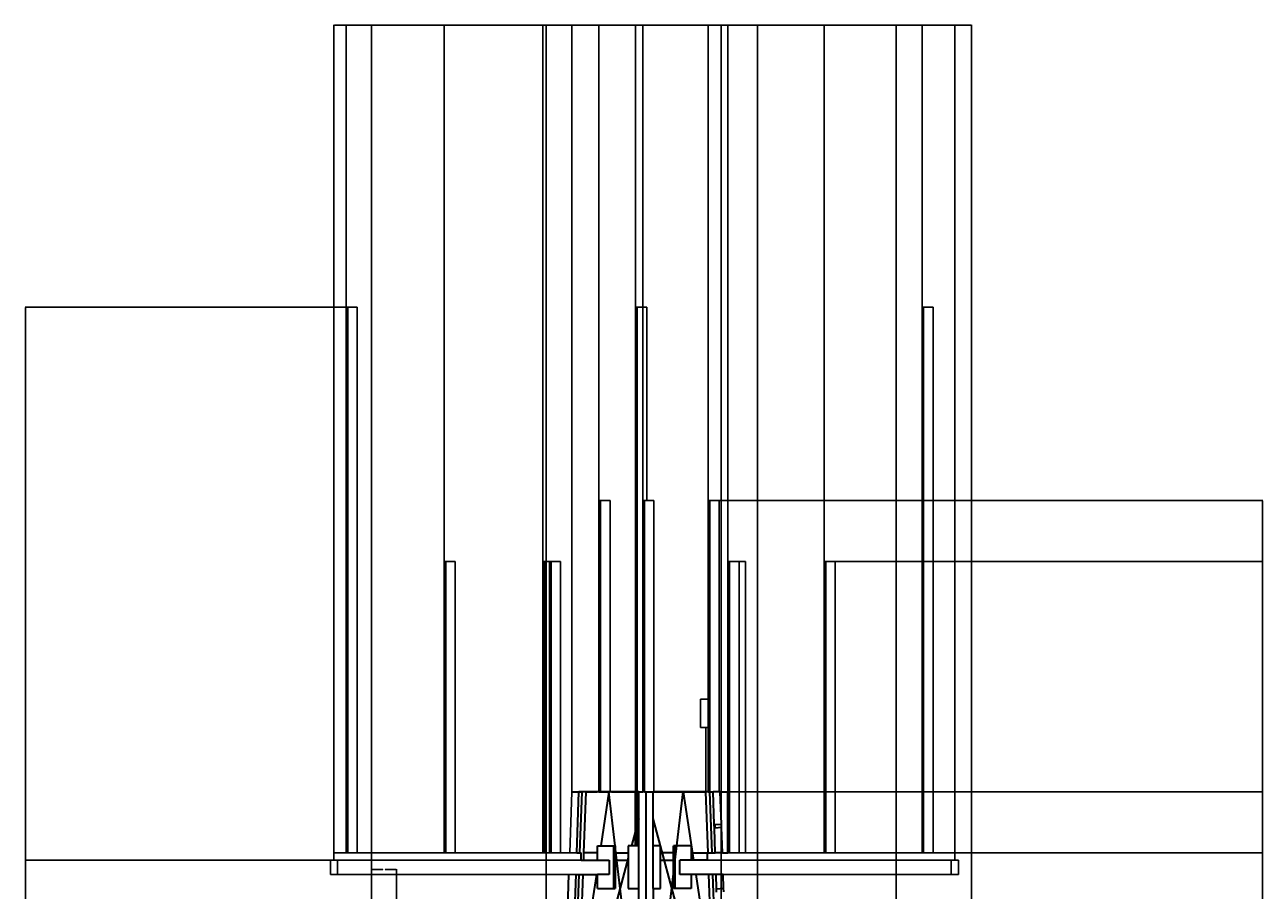
# Model space of a CAD drawing. Units: inches. Extents: x 3780 to 4301, y 1637 to 4224.
# Tile 8 of 8: x 3781 to 4301, y 3860 to 4224. Entities that reach past the tile are written whole.
import ezdxf

# ---------------------------------------------------------------- set-up
doc = ezdxf.new("R2010")
doc.units = ezdxf.units.IN
for name, color, linetype, lineweight in [('A-ANNO-DIMS', 2, 'Continuous', 18), ('E-COMM-ANTN', 4, 'Continuous', 25), ('S-TOWR', 7, 'Continuous', 35)]:
    doc.layers.add(name, color=color, linetype=linetype, lineweight=lineweight)
doc.styles.get("Standard").update_dxf_attribs({"font": 'arial.ttf'})
doc.dimstyles.get("Standard").update_dxf_attribs({"dimtxt": 0.18, "dimasz": 0.18, "dimexe": 0.18, "dimexo": 0.0625, "dimgap": 0.09, "dimtad": 0, "dimtih": 1, "dimtoh": 1, "dimdec": 4, "dimzin": 0, "dimdsep": 46, "dimtxsty": 'Standard', "dimcen": 0.09, "dimadec": 0, "dimazin": 0, "dimtfac": 1, "dimtdec": 4, "dimtofl": 0, "dimtmove": 0, "dimatfit": 3, "dimfxl": 1, "dimtolj": 1, "dimtzin": 0, "dimarcsym": 0})

# ---------------------------------------------------------------- blocks, each defined once
blk = doc.blocks.new('*D8')
at = {"layer": 'A-ANNO-DIMS', "color": 0, "lineweight": -2, "transparency": 16777216}
for p, q in [((3926.23, 3844.62), (3926.23, 3869.04)), ((3926.41, 3868.86), (3931, 3868.86)), ((3936.62, 3868.86), (3932.03, 3868.86)), ((3936.8, 3844.62), (3936.8, 3869.04))]:
    blk.add_line(p, q, dxfattribs=at)
at = {"layer": 'A-ANNO-DIMS', "color": 0, "transparency": 16777216}
for points in [[(3926.41, 3868.89), (3926.41, 3868.83), (3926.23, 3868.86)], [(3936.62, 3868.89), (3936.62, 3868.83), (3936.8, 3868.86)]]:
    blk.add_solid(points, dxfattribs=at)
at = {"layer": 'Defpoints', "color": 0, "transparency": 16777216}
for p in [(3936.8, 3868.86), (3926.23, 3844.56), (3936.8, 3844.56)]:
    blk.add_point(p, dxfattribs=at)
at = {"layer": 'A-ANNO-DIMS', "color": 0, "transparency": 16777216, "insert": (3931.51, 3868.86), "char_height": 0.18, "attachment_point": 5}
blk.add_mtext('\\A1;11 TYP.', dxfattribs=at)
blk = doc.blocks.new('*D11')
at = {"layer": 'A-ANNO-DIMS', "color": 0, "lineweight": -2, "transparency": 16777216}
for p, q in [((3916.19, 4105.28), (3780.66, 4105.28)), ((3780.84, 4105.1), (3780.84, 2930.44)), ((3780.84, 1755.43), (3780.84, 2930.08)), ((3934.09, 1755.25), (3780.66, 1755.25))]:
    blk.add_line(p, q, dxfattribs=at)
at = {"layer": 'A-ANNO-DIMS', "color": 0, "transparency": 16777216}
for points in [[(3780.81, 4105.1), (3780.87, 4105.1), (3780.84, 4105.28)], [(3780.81, 1755.43), (3780.87, 1755.43), (3780.84, 1755.25)]]:
    blk.add_solid(points, dxfattribs=at)
at = {"layer": 'Defpoints', "color": 0, "transparency": 16777216}
for p in [(3780.84, 4105.28), (3916.25, 4105.28), (3934.15, 1755.25)]:
    blk.add_point(p, dxfattribs=at)
at = {"layer": 'A-ANNO-DIMS', "color": 0, "transparency": 16777216, "insert": (3780.84, 2930.26), "char_height": 0.18, "attachment_point": 5}
blk.add_mtext('\\A1;2350', dxfattribs=at)
blk = doc.blocks.new('*D21')
at = {"layer": 'A-ANNO-DIMS', "color": 0, "lineweight": -2, "transparency": 16777216}
for p, q in [((4010.55, 3901.46), (4300.89, 3901.46)), ((4300.71, 3901.28), (4300.71, 3685.65)), ((4300.71, 3469.64), (4300.71, 3685.28)), ((4044.72, 3469.46), (4300.89, 3469.46))]:
    blk.add_line(p, q, dxfattribs=at)
at = {"layer": 'A-ANNO-DIMS', "color": 0, "transparency": 16777216}
for points in [[(4300.68, 3901.28), (4300.74, 3901.28), (4300.71, 3901.46)], [(4300.68, 3469.64), (4300.74, 3469.64), (4300.71, 3469.46)]]:
    blk.add_solid(points, dxfattribs=at)
at = {"layer": 'Defpoints', "color": 0, "transparency": 16777216}
for p in [(4010.49, 3901.46), (4300.71, 3901.46), (4044.66, 3469.46)]:
    blk.add_point(p, dxfattribs=at)
at = {"layer": 'A-ANNO-DIMS', "color": 0, "transparency": 16777216, "insert": (4300.71, 3685.46), "char_height": 0.18, "attachment_point": 5}
blk.add_mtext('\\A1;432', dxfattribs=at)
blk = doc.blocks.new('*D23')
at = {"layer": 'A-ANNO-DIMS', "color": 0, "lineweight": -2, "transparency": 16777216}
for p, q in [((3910.47, 3872.84), (3910.47, 4223.96)), ((3910.65, 4223.78), (4040.69, 4223.78)), ((4171.29, 4223.78), (4041.24, 4223.78)), ((4171.47, 3872.84), (4171.47, 4223.96))]:
    blk.add_line(p, q, dxfattribs=at)
at = {"layer": 'A-ANNO-DIMS', "color": 0, "transparency": 16777216}
for points in [[(3910.65, 4223.81), (3910.65, 4223.75), (3910.47, 4223.78)], [(4171.29, 4223.81), (4171.29, 4223.75), (4171.47, 4223.78)]]:
    blk.add_solid(points, dxfattribs=at)
at = {"layer": 'Defpoints', "color": 0, "transparency": 16777216}
for p in [(4171.47, 4223.78), (3910.47, 3872.78), (4171.47, 3872.78)]:
    blk.add_point(p, dxfattribs=at)
at = {"layer": 'A-ANNO-DIMS', "color": 0, "transparency": 16777216, "insert": (4040.97, 4223.78), "char_height": 0.18, "attachment_point": 5}
blk.add_mtext('\\A1;261', dxfattribs=at)
blk = doc.blocks.new('*D24')
at = {"layer": 'A-ANNO-DIMS', "color": 0, "lineweight": -2, "transparency": 16777216}
for p, q in [((4010.49, 3901.53), (4010.49, 4223.96)), ((4010.67, 4223.78), (4042.96, 4223.78)), ((4075.91, 4223.78), (4043.61, 4223.78)), ((4076.09, 3901.53), (4076.09, 4223.96))]:
    blk.add_line(p, q, dxfattribs=at)
at = {"layer": 'A-ANNO-DIMS', "color": 0, "transparency": 16777216}
for points in [[(4010.67, 4223.81), (4010.67, 4223.75), (4010.49, 4223.78)], [(4075.91, 4223.81), (4075.91, 4223.75), (4076.09, 4223.78)]]:
    blk.add_solid(points, dxfattribs=at)
at = {"layer": 'Defpoints', "color": 0, "transparency": 16777216}
for p in [(4076.09, 4223.78), (4010.49, 3901.46), (4076.09, 3901.46)]:
    blk.add_point(p, dxfattribs=at)
at = {"layer": 'A-ANNO-DIMS', "color": 0, "transparency": 16777216, "insert": (4043.29, 4223.78), "char_height": 0.18, "attachment_point": 5}
blk.add_mtext('\\A1;65.6', dxfattribs=at)
blk = doc.blocks.new('*D25')
at = {"layer": 'A-ANNO-DIMS', "color": 0, "lineweight": -2, "transparency": 16777216}
for p, q in [((3916.19, 4105.28), (3780.66, 4105.28)), ((3780.84, 4105.1), (3780.84, 3989.21)), ((3780.84, 3872.96), (3780.84, 3988.84)), ((3911.9, 3872.78), (3780.66, 3872.78))]:
    blk.add_line(p, q, dxfattribs=at)
at = {"layer": 'A-ANNO-DIMS', "color": 0, "transparency": 16777216}
for points in [[(3780.81, 4105.1), (3780.87, 4105.1), (3780.84, 4105.28)], [(3780.81, 3872.96), (3780.87, 3872.96), (3780.84, 3872.78)]]:
    blk.add_solid(points, dxfattribs=at)
at = {"layer": 'Defpoints', "color": 0, "transparency": 16777216}
for p in [(3780.84, 4105.28), (3916.25, 4105.28), (3911.96, 3872.78)]:
    blk.add_point(p, dxfattribs=at)
at = {"layer": 'A-ANNO-DIMS', "color": 0, "transparency": 16777216, "insert": (3780.84, 3989.03), "char_height": 0.18, "attachment_point": 5}
blk.add_mtext('\\A1;232.5', dxfattribs=at)
blk = doc.blocks.new('*D29')
at = {"layer": 'A-ANNO-DIMS', "color": 0, "lineweight": -2, "transparency": 16777216}
for p, q in [((3916.19, 4105.28), (3780.66, 4105.28)), ((3780.84, 4105.1), (3780.84, 3898.77)), ((3780.84, 3692.09), (3780.84, 3898.41)), ((3926.17, 3691.91), (3780.66, 3691.91))]:
    blk.add_line(p, q, dxfattribs=at)
at = {"layer": 'A-ANNO-DIMS', "color": 0, "transparency": 16777216}
for points in [[(3780.81, 4105.1), (3780.87, 4105.1), (3780.84, 4105.28)], [(3780.81, 3692.09), (3780.87, 3692.09), (3780.84, 3691.91)]]:
    blk.add_solid(points, dxfattribs=at)
at = {"layer": 'Defpoints', "color": 0, "transparency": 16777216}
for p in [(3780.84, 4105.28), (3916.25, 4105.28), (3926.23, 3691.91)]:
    blk.add_point(p, dxfattribs=at)
at = {"layer": 'A-ANNO-DIMS', "color": 0, "transparency": 16777216, "insert": (3780.84, 3898.59), "char_height": 0.18, "attachment_point": 5}
blk.add_mtext('\\A1;413.4', dxfattribs=at)
blk = doc.blocks.new('*D30')
at = {"layer": 'A-ANNO-DIMS', "color": 0, "lineweight": -2, "transparency": 16777216}
for p, q in [((3915.57, 4105.34), (3915.57, 4223.96)), ((3915.75, 4223.78), (3976.03, 4223.78)), ((4037.08, 4223.78), (3976.8, 4223.78)), ((4037.26, 4105.34), (4037.26, 4223.96))]:
    blk.add_line(p, q, dxfattribs=at)
at = {"layer": 'A-ANNO-DIMS', "color": 0, "transparency": 16777216}
for points in [[(3915.75, 4223.81), (3915.75, 4223.75), (3915.57, 4223.78)], [(4037.08, 4223.81), (4037.08, 4223.75), (4037.26, 4223.78)]]:
    blk.add_solid(points, dxfattribs=at)
at = {"layer": 'Defpoints', "color": 0, "transparency": 16777216}
for p in [(4037.26, 4223.78), (3915.57, 4105.28), (4037.26, 4105.28)]:
    blk.add_point(p, dxfattribs=at)
at = {"layer": 'A-ANNO-DIMS', "color": 0, "transparency": 16777216, "insert": (3976.41, 4223.78), "char_height": 0.18, "attachment_point": 5}
blk.add_mtext('\\A1;121.7', dxfattribs=at)
blk = doc.blocks.new('*D31')
at = {"layer": 'A-ANNO-DIMS', "color": 0, "lineweight": -2, "transparency": 16777216}
for p, q in [((4037.26, 4105.34), (4037.26, 4223.96)), ((4037.44, 4223.78), (4097.08, 4223.78)), ((4157.48, 4223.78), (4097.85, 4223.78)), ((4157.66, 4105.34), (4157.66, 4223.96))]:
    blk.add_line(p, q, dxfattribs=at)
at = {"layer": 'A-ANNO-DIMS', "color": 0, "transparency": 16777216}
for points in [[(4037.44, 4223.81), (4037.44, 4223.75), (4037.26, 4223.78)], [(4157.48, 4223.81), (4157.48, 4223.75), (4157.66, 4223.78)]]:
    blk.add_solid(points, dxfattribs=at)
at = {"layer": 'Defpoints', "color": 0, "transparency": 16777216}
for p in [(4157.66, 4223.78), (4037.26, 4105.28), (4157.66, 4105.28)]:
    blk.add_point(p, dxfattribs=at)
at = {"layer": 'A-ANNO-DIMS', "color": 0, "transparency": 16777216, "insert": (4097.46, 4223.78), "char_height": 0.18, "attachment_point": 5}
blk.add_mtext('\\A1;120.4', dxfattribs=at)
blk = doc.blocks.new('*D32')
at = {"layer": 'A-ANNO-DIMS', "color": 0, "lineweight": -2, "transparency": 16777216}
for p, q in [((3956.8, 3998.37), (3956.8, 4223.96)), ((3956.98, 4223.78), (3977.08, 4223.78)), ((3998.11, 4223.78), (3978.01, 4223.78)), ((3998.29, 3998.37), (3998.29, 4223.96))]:
    blk.add_line(p, q, dxfattribs=at)
at = {"layer": 'A-ANNO-DIMS', "color": 0, "transparency": 16777216}
for points in [[(3956.98, 4223.81), (3956.98, 4223.75), (3956.8, 4223.78)], [(3998.11, 4223.81), (3998.11, 4223.75), (3998.29, 4223.78)]]:
    blk.add_solid(points, dxfattribs=at)
at = {"layer": 'Defpoints', "color": 0, "transparency": 16777216}
for p in [(3998.29, 4223.78), (3956.8, 3998.31), (3998.29, 3998.31)]:
    blk.add_point(p, dxfattribs=at)
at = {"layer": 'A-ANNO-DIMS', "color": 0, "transparency": 16777216, "insert": (3977.55, 4223.78), "char_height": 0.18, "attachment_point": 5}
blk.add_mtext('\\A1;41.484', dxfattribs=at)
blk = doc.blocks.new('*D33')
at = {"layer": 'A-ANNO-DIMS', "color": 0, "lineweight": -2, "transparency": 16777216}
for p, q in [((3998.29, 3998.37), (3998.29, 4223.96)), ((3998.47, 4223.78), (4036.87, 4223.78)), ((4075.91, 4223.78), (4037.51, 4223.78)), ((4076.09, 3998.37), (4076.09, 4223.96))]:
    blk.add_line(p, q, dxfattribs=at)
at = {"layer": 'A-ANNO-DIMS', "color": 0, "transparency": 16777216}
for points in [[(3998.47, 4223.81), (3998.47, 4223.75), (3998.29, 4223.78)], [(4075.91, 4223.81), (4075.91, 4223.75), (4076.09, 4223.78)]]:
    blk.add_solid(points, dxfattribs=at)
at = {"layer": 'Defpoints', "color": 0, "transparency": 16777216}
for p in [(4076.09, 4223.78), (3998.29, 3998.31), (4076.09, 3998.31)]:
    blk.add_point(p, dxfattribs=at)
at = {"layer": 'A-ANNO-DIMS', "color": 0, "transparency": 16777216, "insert": (4037.19, 4223.78), "char_height": 0.18, "attachment_point": 5}
blk.add_mtext('\\A1;77.8', dxfattribs=at)
blk = doc.blocks.new('*D34')
at = {"layer": 'A-ANNO-DIMS', "color": 0, "lineweight": -2, "transparency": 16777216}
for p, q in [((4076.09, 3998.37), (4076.09, 4223.96)), ((4076.27, 4223.78), (4095.84, 4223.78)), ((4116.34, 4223.78), (4096.77, 4223.78)), ((4116.52, 3998.37), (4116.52, 4223.96))]:
    blk.add_line(p, q, dxfattribs=at)
at = {"layer": 'A-ANNO-DIMS', "color": 0, "transparency": 16777216}
for points in [[(4076.27, 4223.81), (4076.27, 4223.75), (4076.09, 4223.78)], [(4116.34, 4223.81), (4116.34, 4223.75), (4116.52, 4223.78)]]:
    blk.add_solid(points, dxfattribs=at)
at = {"layer": 'Defpoints', "color": 0, "transparency": 16777216}
for p in [(4116.52, 4223.78), (4076.09, 3998.31), (4116.52, 3998.31)]:
    blk.add_point(p, dxfattribs=at)
at = {"layer": 'A-ANNO-DIMS', "color": 0, "transparency": 16777216, "insert": (4096.3, 4223.78), "char_height": 0.18, "attachment_point": 5}
blk.add_mtext('\\A1;40.425', dxfattribs=at)
blk = doc.blocks.new('*D35')
at = {"layer": 'A-ANNO-DIMS', "color": 0, "lineweight": -2, "transparency": 16777216}
for p, q in [((4021.84, 4024.06), (4021.84, 4223.96)), ((4022.02, 4223.78), (4030.67, 4223.78)), ((4040.1, 4223.78), (4031.44, 4223.78)), ((4040.28, 4024.06), (4040.28, 4223.96))]:
    blk.add_line(p, q, dxfattribs=at)
at = {"layer": 'A-ANNO-DIMS', "color": 0, "transparency": 16777216}
for points in [[(4022.02, 4223.81), (4022.02, 4223.75), (4021.84, 4223.78)], [(4040.1, 4223.81), (4040.1, 4223.75), (4040.28, 4223.78)]]:
    blk.add_solid(points, dxfattribs=at)
at = {"layer": 'Defpoints', "color": 0, "transparency": 16777216}
for p in [(4040.28, 4223.78), (4021.84, 4024), (4040.28, 4024)]:
    blk.add_point(p, dxfattribs=at)
at = {"layer": 'A-ANNO-DIMS', "color": 0, "transparency": 16777216, "insert": (4031.06, 4223.78), "char_height": 0.18, "attachment_point": 5}
blk.add_mtext('\\A1;18.44', dxfattribs=at)
blk = doc.blocks.new('*D36')
at = {"layer": 'A-ANNO-DIMS', "color": 0, "lineweight": -2, "transparency": 16777216}
for p, q in [((4040.28, 4024.06), (4040.28, 4223.96)), ((4040.46, 4223.78), (4053.56, 4223.78)), ((4067.58, 4223.78), (4054.49, 4223.78)), ((4067.76, 4024.06), (4067.76, 4223.96))]:
    blk.add_line(p, q, dxfattribs=at)
at = {"layer": 'A-ANNO-DIMS', "color": 0, "transparency": 16777216}
for points in [[(4040.46, 4223.81), (4040.46, 4223.75), (4040.28, 4223.78)], [(4067.58, 4223.81), (4067.58, 4223.75), (4067.76, 4223.78)]]:
    blk.add_solid(points, dxfattribs=at)
at = {"layer": 'Defpoints', "color": 0, "transparency": 16777216}
for p in [(4067.76, 4223.78), (4040.28, 4024), (4067.76, 4024)]:
    blk.add_point(p, dxfattribs=at)
at = {"layer": 'A-ANNO-DIMS', "color": 0, "transparency": 16777216, "insert": (4054.02, 4223.78), "char_height": 0.18, "attachment_point": 5}
blk.add_mtext('\\A1;27.487', dxfattribs=at)
blk = doc.blocks.new('*D37')
at = {"layer": 'A-ANNO-DIMS', "color": 0, "lineweight": -2, "transparency": 16777216}
for p, q in [((4121.27, 3998.31), (4300.89, 3998.31)), ((4300.71, 3998.13), (4300.71, 3937.22)), ((4300.71, 3875.96), (4300.71, 3936.86)), ((4121.27, 3875.78), (4300.89, 3875.78))]:
    blk.add_line(p, q, dxfattribs=at)
at = {"layer": 'A-ANNO-DIMS', "color": 0, "transparency": 16777216}
for points in [[(4300.68, 3998.13), (4300.74, 3998.13), (4300.71, 3998.31)], [(4300.68, 3875.96), (4300.74, 3875.96), (4300.71, 3875.78)]]:
    blk.add_solid(points, dxfattribs=at)
at = {"layer": 'Defpoints', "color": 0, "transparency": 16777216}
for p in [(4121.2, 3998.31), (4300.71, 3998.31), (4121.2, 3875.78)]:
    blk.add_point(p, dxfattribs=at)
at = {"layer": 'A-ANNO-DIMS', "color": 0, "transparency": 16777216, "insert": (4300.71, 3937.04), "char_height": 0.18, "attachment_point": 5}
blk.add_mtext('\\A1;122.53', dxfattribs=at)
blk = doc.blocks.new('*D38')
at = {"layer": 'A-ANNO-DIMS', "color": 0, "lineweight": -2, "transparency": 16777216}
for p, q in [((4072.51, 4024), (4300.89, 4024)), ((4300.71, 4023.82), (4300.71, 3950.07)), ((4300.71, 3875.96), (4300.71, 3949.7)), ((4070.82, 3875.78), (4300.89, 3875.78))]:
    blk.add_line(p, q, dxfattribs=at)
at = {"layer": 'A-ANNO-DIMS', "color": 0, "transparency": 16777216}
for points in [[(4300.68, 4023.82), (4300.74, 4023.82), (4300.71, 4024)], [(4300.68, 3875.96), (4300.74, 3875.96), (4300.71, 3875.78)]]:
    blk.add_solid(points, dxfattribs=at)
at = {"layer": 'Defpoints', "color": 0, "transparency": 16777216}
for p in [(4072.45, 4024), (4300.71, 4024), (4070.75, 3875.78)]:
    blk.add_point(p, dxfattribs=at)
at = {"layer": 'A-ANNO-DIMS', "color": 0, "transparency": 16777216, "insert": (4300.71, 3949.89), "char_height": 0.18, "attachment_point": 5}
blk.add_mtext('\\A1;148.22', dxfattribs=at)
blk = doc.blocks.new('*D39')
at = {"layer": 'A-ANNO-DIMS', "color": 0, "lineweight": -2, "transparency": 16777216}
for p, q in [((3926.23, 3835.97), (3926.23, 4223.96)), ((3926.41, 4223.78), (3962.66, 4223.78)), ((3999.55, 4223.78), (3963.31, 4223.78)), ((3999.73, 3835.97), (3999.73, 4223.96))]:
    blk.add_line(p, q, dxfattribs=at)
at = {"layer": 'A-ANNO-DIMS', "color": 0, "transparency": 16777216}
for points in [[(3926.41, 4223.81), (3926.41, 4223.75), (3926.23, 4223.78)], [(3999.55, 4223.81), (3999.55, 4223.75), (3999.73, 4223.78)]]:
    blk.add_solid(points, dxfattribs=at)
at = {"layer": 'Defpoints', "color": 0, "transparency": 16777216}
for p in [(3999.73, 4223.78), (3926.23, 3835.91), (3999.73, 3835.91)]:
    blk.add_point(p, dxfattribs=at)
at = {"layer": 'A-ANNO-DIMS', "color": 0, "transparency": 16777216, "insert": (3962.98, 4223.78), "char_height": 0.18, "attachment_point": 5}
blk.add_mtext('\\A1;73.5', dxfattribs=at)
blk = doc.blocks.new('*D40')
at = {"layer": 'A-ANNO-DIMS', "color": 0, "lineweight": -2, "transparency": 16777216}
for p, q in [((3999.73, 3835.97), (3999.73, 4223.96)), ((3999.91, 4223.78), (4036.16, 4223.78)), ((4073.05, 4223.78), (4036.81, 4223.78)), ((4073.23, 3835.97), (4073.23, 4223.96))]:
    blk.add_line(p, q, dxfattribs=at)
at = {"layer": 'A-ANNO-DIMS', "color": 0, "transparency": 16777216}
for points in [[(3999.91, 4223.81), (3999.91, 4223.75), (3999.73, 4223.78)], [(4073.05, 4223.81), (4073.05, 4223.75), (4073.23, 4223.78)]]:
    blk.add_solid(points, dxfattribs=at)
at = {"layer": 'Defpoints', "color": 0, "transparency": 16777216}
for p in [(4073.23, 4223.78), (3999.73, 3835.91), (4073.23, 3835.91)]:
    blk.add_point(p, dxfattribs=at)
at = {"layer": 'A-ANNO-DIMS', "color": 0, "transparency": 16777216, "insert": (4036.48, 4223.78), "char_height": 0.18, "attachment_point": 5}
blk.add_mtext('\\A1;73.5', dxfattribs=at)
blk = doc.blocks.new('*D41')
at = {"layer": 'A-ANNO-DIMS', "color": 0, "lineweight": -2, "transparency": 16777216}
for p, q in [((4073.23, 3835.97), (4073.23, 4223.96)), ((4073.41, 4223.78), (4109.66, 4223.78)), ((4146.55, 4223.78), (4110.31, 4223.78)), ((4146.73, 3835.97), (4146.73, 4223.96))]:
    blk.add_line(p, q, dxfattribs=at)
at = {"layer": 'A-ANNO-DIMS', "color": 0, "transparency": 16777216}
for points in [[(4073.41, 4223.81), (4073.41, 4223.75), (4073.23, 4223.78)], [(4146.55, 4223.81), (4146.55, 4223.75), (4146.73, 4223.78)]]:
    blk.add_solid(points, dxfattribs=at)
at = {"layer": 'Defpoints', "color": 0, "transparency": 16777216}
for p in [(4146.73, 4223.78), (4073.23, 3835.91), (4146.73, 3835.91)]:
    blk.add_point(p, dxfattribs=at)
at = {"layer": 'A-ANNO-DIMS', "color": 0, "transparency": 16777216, "insert": (4109.98, 4223.78), "char_height": 0.18, "attachment_point": 5}
blk.add_mtext('\\A1;73.5', dxfattribs=at)
blk = doc.blocks.new('*D48')
at = {"layer": 'A-ANNO-DIMS', "color": 0, "lineweight": -2, "transparency": 16777216}
for p, q in [((3926.23, 3245.63), (3926.23, 4223.96)), ((3926.41, 4223.78), (3962.66, 4223.78)), ((3999.55, 4223.78), (3963.31, 4223.78)), ((3999.73, 3245.63), (3999.73, 4223.96))]:
    blk.add_line(p, q, dxfattribs=at)
at = {"layer": 'A-ANNO-DIMS', "color": 0, "transparency": 16777216}
for points in [[(3926.41, 4223.81), (3926.41, 4223.75), (3926.23, 4223.78)], [(3999.55, 4223.81), (3999.55, 4223.75), (3999.73, 4223.78)]]:
    blk.add_solid(points, dxfattribs=at)
at = {"layer": 'Defpoints', "color": 0, "transparency": 16777216}
for p in [(3999.73, 4223.78), (3926.23, 3245.56), (3999.73, 3245.56)]:
    blk.add_point(p, dxfattribs=at)
at = {"layer": 'A-ANNO-DIMS', "color": 0, "transparency": 16777216, "insert": (3962.98, 4223.78), "char_height": 0.18, "attachment_point": 5}
blk.add_mtext('\\A1;73.5', dxfattribs=at)
blk = doc.blocks.new('*D49')
at = {"layer": 'A-ANNO-DIMS', "color": 0, "lineweight": -2, "transparency": 16777216}
for p, q in [((3999.73, 3245.63), (3999.73, 4223.96)), ((3999.91, 4223.78), (4036.16, 4223.78)), ((4073.05, 4223.78), (4036.81, 4223.78)), ((4073.23, 3245.63), (4073.23, 4223.96))]:
    blk.add_line(p, q, dxfattribs=at)
at = {"layer": 'A-ANNO-DIMS', "color": 0, "transparency": 16777216}
for points in [[(3999.91, 4223.81), (3999.91, 4223.75), (3999.73, 4223.78)], [(4073.05, 4223.81), (4073.05, 4223.75), (4073.23, 4223.78)]]:
    blk.add_solid(points, dxfattribs=at)
at = {"layer": 'Defpoints', "color": 0, "transparency": 16777216}
for p in [(4073.23, 4223.78), (3999.73, 3245.56), (4073.23, 3245.56)]:
    blk.add_point(p, dxfattribs=at)
at = {"layer": 'A-ANNO-DIMS', "color": 0, "transparency": 16777216, "insert": (4036.48, 4223.78), "char_height": 0.18, "attachment_point": 5}
blk.add_mtext('\\A1;73.5', dxfattribs=at)
blk = doc.blocks.new('*D50')
at = {"layer": 'A-ANNO-DIMS', "color": 0, "lineweight": -2, "transparency": 16777216}
for p, q in [((4073.23, 3245.63), (4073.23, 4223.96)), ((4073.41, 4223.78), (4109.66, 4223.78)), ((4146.55, 4223.78), (4110.31, 4223.78)), ((4146.73, 3245.63), (4146.73, 4223.96))]:
    blk.add_line(p, q, dxfattribs=at)
at = {"layer": 'A-ANNO-DIMS', "color": 0, "transparency": 16777216}
for points in [[(4073.41, 4223.81), (4073.41, 4223.75), (4073.23, 4223.78)], [(4146.55, 4223.81), (4146.55, 4223.75), (4146.73, 4223.78)]]:
    blk.add_solid(points, dxfattribs=at)
at = {"layer": 'Defpoints', "color": 0, "transparency": 16777216}
for p in [(4146.73, 4223.78), (4073.23, 3245.56), (4146.73, 3245.56)]:
    blk.add_point(p, dxfattribs=at)
at = {"layer": 'A-ANNO-DIMS', "color": 0, "transparency": 16777216, "insert": (4109.98, 4223.78), "char_height": 0.18, "attachment_point": 5}
blk.add_mtext('\\A1;73.5', dxfattribs=at)
blk = doc.blocks.new('*D59')
at = {"layer": 'A-ANNO-DIMS', "color": 0, "lineweight": -2, "transparency": 16777216}
for p, q in [((4088.55, 3352.58), (4088.55, 4223.96)), ((4088.73, 4223.78), (4133.13, 4223.78)), ((4178.28, 4223.78), (4133.88, 4223.78)), ((4178.46, 3329.55), (4178.46, 4223.96))]:
    blk.add_line(p, q, dxfattribs=at)
at = {"layer": 'A-ANNO-DIMS', "color": 0, "transparency": 16777216}
for points in [[(4088.73, 4223.81), (4088.73, 4223.75), (4088.55, 4223.78)], [(4178.28, 4223.81), (4178.28, 4223.75), (4178.46, 4223.78)]]:
    blk.add_solid(points, dxfattribs=at)
at = {"layer": 'Defpoints', "color": 0, "transparency": 16777216}
for p in [(4178.46, 4223.78), (4088.55, 3352.51), (4178.46, 3329.49)]:
    blk.add_point(p, dxfattribs=at)
at = {"layer": 'A-ANNO-DIMS', "color": 0, "transparency": 16777216, "insert": (4133.51, 4223.78), "char_height": 0.18, "attachment_point": 5}
blk.add_mtext('\\A1;89.91', dxfattribs=at)

msp = doc.modelspace()

# ---------------------------------------------------------------- linework, layer by layer
at = {"layer": 'E-COMM-ANTN'}
for p, q in [((3915.5655, 3875.7769), (3915.5655, 4105.2769)), ((3915.5655, 4105.2769), (3916.252, 4105.2769)), ((3916.252, 3875.7769), (3916.252, 4105.2769)), ((3916.252, 4105.2769), (3920.253, 4105.2769)), ((3920.253, 3875.7769), (3920.253, 4105.2769)), ((4037.2616, 3901.4644), (4037.2616, 4105.2769)), ((4037.9481, 4105.2769), (4037.2616, 4105.2769)), ((4037.9481, 3901.4644), (4037.9481, 4105.2769)), ((4041.9491, 4105.2769), (4037.9481, 4105.2769)), ((4041.9491, 4023.9957), (4041.9491, 4105.2769)), ((4157.6646, 3875.7769), (4157.6646, 4105.2769)), ((4157.6646, 4105.2769), (4158.3511, 4105.2769)), ((4158.3511, 3875.7769), (4158.3511, 4105.2769)), ((4162.3521, 4105.2769), (4158.3511, 4105.2769)), ((4162.3521, 3875.7769), (4162.3521, 4105.2769)), ((4021.8362, 3901.4644), (4021.8362, 4023.9957)), ((4022.5227, 4023.9957), (4021.8362, 4023.9957)), ((4022.5227, 3901.4644), (4022.5227, 4023.9957)), ((4026.5237, 4023.9957), (4022.5227, 4023.9957)), ((4026.5237, 3901.4644), (4026.5237, 4023.9957)), ((4040.2769, 3901.4644), (4040.2769, 4023.9957)), ((4040.9633, 4023.9957), (4040.2769, 4023.9957)), ((4040.9633, 3901.4644), (4040.9633, 4023.9957)), ((4040.9633, 4023.9957), (4041.9491, 4023.9957)), ((4044.9644, 4023.9957), (4041.9491, 4023.9957)), ((4044.9644, 3901.4644), (4044.9644, 4023.9957)), ((4067.7636, 3940.4644), (4067.7636, 4023.9957)), ((4067.7636, 4023.9957), (4068.4501, 4023.9957)), ((4068.4501, 3901.4644), (4068.4501, 4023.9957)), ((4072.4511, 4023.9957), (4068.4501, 4023.9957)), ((4072.4511, 3901.4644), (4072.4511, 4023.9957)), ((3956.8041, 3875.7769), (3956.8041, 3998.3082)), ((3956.8041, 3998.3082), (3957.4906, 3998.3082)), ((3957.4906, 3875.7769), (3957.4906, 3998.3082)), ((3961.4916, 3998.3082), (3957.4906, 3998.3082)), ((3961.4916, 3875.7769), (3961.4916, 3998.3082)), ((3998.2885, 3875.7769), (3998.2885, 3998.3082)), ((3998.975, 3998.3082), (3998.2885, 3998.3082)), ((3998.975, 3875.7769), (3998.975, 3998.3082)), ((4001.0899, 3998.3082), (3998.975, 3998.3082)), ((4001.0899, 3875.7769), (4001.0899, 3998.3082)), ((4001.7764, 3998.3082), (4001.0899, 3998.3082)), ((4001.7764, 3875.7769), (4001.7764, 3998.3082)), ((4005.7774, 3998.3082), (4001.7764, 3998.3082)), ((4005.7774, 3875.7769), (4005.7774, 3998.3082)), ((4076.0906, 3901.4644), (4076.0906, 3998.3082)), ((4076.777, 3998.3082), (4076.0906, 3998.3082)), ((4076.777, 3875.7769), (4076.777, 3998.3082)), ((4080.7781, 3998.3082), (4076.777, 3998.3082)), ((4080.7781, 3875.7769), (4080.7781, 3998.3082)), ((4080.7781, 3998.3082), (4083.4281, 3998.3082)), ((4083.4281, 3875.7769), (4083.4281, 3998.3082)), ((4116.5154, 3875.7769), (4116.5154, 3998.3082)), ((4117.2019, 3998.3082), (4116.5154, 3998.3082)), ((4117.2019, 3875.7769), (4117.2019, 3998.3082)), ((4121.2029, 3998.3082), (4117.2019, 3998.3082)), ((4121.2029, 3875.7769), (4121.2029, 3998.3082)), ((4064.5755, 3928.4644), (4064.5755, 3940.4644)), ((4067.7636, 3940.4644), (4064.5755, 3940.4644)), ((4067.7636, 3928.4644), (4067.7636, 3940.4644)), ((4066.8391, 3928.4644), (4064.5755, 3928.4644)), ((4066.8391, 3901.4644), (4066.8391, 3928.4644)), ((4066.8391, 3928.4644), (4067.7636, 3928.4644)), ((4067.7636, 3901.4644), (4067.7636, 3928.4644)), ((4009.5717, 3875.7769), (4010.4853, 3901.4644)), ((3910.4676, 3872.7769), (3910.4676, 3875.7769)), ((3910.4676, 3875.7769), (3915.5655, 3875.7769)), ((3910.6912, 3875.7769), (3910.4676, 3875.7769)), ((3911.3468, 3875.7769), (3910.6912, 3875.7769)), ((3912.3897, 3875.7769), (3911.3468, 3875.7769)), ((3913.7488, 3875.7769), (3912.3897, 3875.7769)), ((3915.3316, 3875.7769), (3913.7488, 3875.7769)), ((3917.0301, 3875.7769), (3915.3316, 3875.7769)), ((3915.5655, 3875.7769), (3916.252, 3875.7769)), ((3916.252, 3875.7769), (3920.253, 3875.7769)), ((3920.253, 3875.7769), (3956.8041, 3875.7769)), ((3957.4906, 3875.7769), (3956.8041, 3875.7769)), ((3961.4916, 3875.7769), (3957.4906, 3875.7769)), ((3998.2885, 3875.7769), (3961.4916, 3875.7769)), ((3998.975, 3875.7769), (3998.2885, 3875.7769)), ((3998.975, 3875.7769), (4001.0899, 3875.7769)), ((4001.0899, 3875.7769), (4001.7764, 3875.7769)), ((4005.7774, 3875.7769), (4001.7764, 3875.7769)), ((4009.5717, 3875.7769), (4005.7774, 3875.7769)), ((4012.5717, 3875.7769), (4009.5717, 3875.7769)), ((4076.777, 3875.7769), (4080.7781, 3875.7769)), ((4080.7781, 3875.7769), (4083.4281, 3875.7769)), ((4083.4281, 3875.7769), (4116.5154, 3875.7769)), ((4117.2019, 3875.7769), (4116.5154, 3875.7769)), ((4117.2019, 3875.7769), (4121.2029, 3875.7769)), ((4121.2029, 3875.7769), (4157.6646, 3875.7769)), ((4157.6646, 3875.7769), (4158.3511, 3875.7769)), ((4158.3511, 3875.7769), (4162.3521, 3875.7769)), ((4171.4676, 3875.7769), (4162.3521, 3875.7769)), ((4171.4676, 3872.7769), (4171.4676, 3875.7769)), ((3908.976, 3872.7769), (3910.4676, 3872.7769)), ((3908.976, 3866.7769), (3908.976, 3872.7769)), ((3910.4676, 3872.7769), (3911.9591, 3872.7769)), ((3911.9591, 3872.7769), (3911.9591, 3866.7769)), ((4014.3906, 3872.7769), (3911.9591, 3872.7769)), ((4067.5445, 3872.7769), (4169.976, 3872.7769)), ((4169.976, 3872.7769), (4171.4676, 3872.7769)), ((4169.976, 3866.7769), (4169.976, 3872.7769)), ((4172.9591, 3872.7769), (4171.4676, 3872.7769)), ((4172.9591, 3872.7769), (4172.9591, 3866.7769)), ((3911.9591, 3866.7769), (3908.976, 3866.7769)), ((3911.9591, 3866.7769), (4009.2516, 3866.7769)), ((4009.2516, 3866.7769), (4012.2516, 3866.7769)), ((4169.976, 3866.7769), (4074.0728, 3866.7769)), ((4172.9591, 3866.7769), (4169.976, 3866.7769))]:
    msp.add_line(p, q, dxfattribs=at)
at = {"layer": 'S-TOWR'}
for p, q in [((4010.4853, 3901.4644), (4013.4853, 3901.4644)), ((4012.5717, 3875.7769), (4013.4853, 3901.4644)), ((4013.4853, 3901.4644), (4014.7843, 3901.4644)), ((4026.0737, 3901.4644), (4013.4853, 3901.4644)), ((4013.8707, 3875.7769), (4014.7843, 3901.4644)), ((4016.4853, 3901.4644), (4014.7843, 3901.4644)), ((4015.5717, 3875.7769), (4016.4853, 3901.4644)), ((4016.4853, 3901.4644), (4021.1583, 3901.4644)), ((4021.8362, 3901.4644), (4017.6175, 3901.4644)), ((4021.8362, 3901.4644), (4022.5227, 3901.4644)), ((4022.5227, 3901.4644), (4026.5237, 3901.4644)), ((4026.0737, 3901.4644), (4022.6224, 3878.7769)), ((4028.7182, 3878.7769), (4026.0737, 3901.4644)), ((4038.6622, 3901.4644), (4026.0737, 3901.4644)), ((4030.7425, 3901.4644), (4026.5237, 3901.4644)), ((4027.2016, 3901.4644), (4038.6622, 3901.4644)), ((4036.0581, 3901.4644), (4037.2616, 3901.4644)), ((4037.2616, 3878.7769), (4037.2616, 3901.4644)), ((4037.2616, 3901.4644), (4037.9481, 3901.4644)), ((4037.9481, 3878.7769), (4037.9481, 3901.4644)), ((4038.6622, 3901.4644), (4037.9481, 3901.4644)), ((4038.6622, 3878.7769), (4038.6622, 3901.4644)), ((4038.6622, 3901.4644), (4040.2769, 3901.4644)), ((4040.9633, 3901.4644), (4040.2769, 3901.4644)), ((4040.9633, 3901.4644), (4041.6622, 3901.4644)), ((4041.6622, 3763.5582), (4041.6622, 3901.4644)), ((4041.6622, 3901.4644), (4044.6622, 3901.4644)), ((4044.6622, 3878.7769), (4044.6622, 3901.4644)), ((4044.6622, 3901.4644), (4044.9644, 3901.4644)), ((4057.2507, 3901.4644), (4044.6622, 3901.4644)), ((4044.6622, 3793.4644), (4057.2507, 3901.4644)), ((4044.6622, 3901.4644), (4066.8391, 3901.4644)), ((4049.1831, 3901.4644), (4044.9644, 3901.4644)), ((4065.0034, 3901.4644), (4057.2507, 3901.4644)), ((4057.2507, 3901.4644), (4061.6148, 3872.7769)), ((4066.8391, 3901.4644), (4063.5449, 3901.4644)), ((4067.7527, 3875.7769), (4066.8391, 3901.4644)), ((4067.7636, 3901.4644), (4066.8391, 3901.4644)), ((4067.7636, 3901.4644), (4068.4501, 3901.4644)), ((4068.4501, 3901.4644), (4068.5401, 3901.4644)), ((4069.4537, 3875.7769), (4068.5401, 3901.4644)), ((4068.5401, 3901.4644), (4069.8391, 3901.4644)), ((4070.3274, 3887.7359), (4069.8391, 3901.4644)), ((4072.4511, 3901.4644), (4069.8391, 3901.4644)), ((4072.8391, 3901.4644), (4072.4511, 3901.4644)), ((4073.3198, 3887.949), (4072.8391, 3901.4644)), ((4072.8391, 3901.4644), (4076.0906, 3901.4644)), ((4076.0906, 3875.7769), (4076.0906, 3901.4644)), ((4038.6622, 3890.299), (4035.5664, 3878.7769)), ((4070.6803, 3793.4644), (4044.6622, 3890.299)), ((4070.3274, 3887.7359), (4070.7283, 3887.7645)), ((4070.3807, 3886.2372), (4070.3274, 3887.7359)), ((4070.7816, 3886.2657), (4070.3807, 3886.2372)), ((4070.7527, 3875.7769), (4070.3807, 3886.2372)), ((4070.7283, 3887.7645), (4073.3198, 3887.949)), ((4070.7816, 3886.2657), (4070.7283, 3887.7645)), ((4073.3731, 3886.4502), (4070.7816, 3886.2657)), ((4073.3731, 3886.4502), (4073.3198, 3887.949)), ((4073.7527, 3875.7769), (4073.3731, 3886.4502)), ((4021.2379, 3878.7769), (4027.9879, 3878.7769)), ((4021.2379, 3875.7769), (4021.2379, 3878.7769)), ((4027.9879, 3878.7769), (4027.9879, 3860.7769)), ((4027.9879, 3878.7769), (4028.7541, 3878.7769)), ((4028.7541, 3878.7769), (4028.7541, 3875.7769)), ((4038.6622, 3793.4644), (4028.7541, 3878.4687)), ((4037.2616, 3878.7769), (4034.2176, 3878.7769)), ((4034.2176, 3878.7769), (4034.2176, 3875.7769)), ((4037.9481, 3878.7769), (4037.2616, 3878.7769)), ((4038.6622, 3878.7769), (4037.9481, 3878.7769)), ((4038.6622, 3860.7769), (4038.6622, 3878.7769)), ((4047.7176, 3878.7769), (4044.6622, 3878.7769)), ((4044.6622, 3860.7769), (4044.6622, 3878.7769)), ((4047.7176, 3875.7769), (4047.7176, 3878.7769)), ((4053.9472, 3878.7769), (4053.181, 3878.7769)), ((4053.181, 3875.7769), (4053.181, 3878.7769)), ((4053.9472, 3860.7769), (4053.9472, 3878.7769)), ((4060.6972, 3878.7769), (4053.9472, 3878.7769)), ((4060.6972, 3878.7769), (4060.6972, 3875.7769)), ((4012.5717, 3875.7769), (4013.8707, 3875.7769)), ((4034.2176, 3873.7569), (4012.6441, 3793.4644)), ((4013.8707, 3875.7769), (4014.3906, 3875.7769)), ((4014.3906, 3872.7769), (4014.3906, 3875.7769)), ((4015.465, 3872.7769), (4015.5717, 3875.7769)), ((4021.2379, 3875.7769), (4015.5717, 3875.7769)), ((4021.2379, 3872.7769), (4021.2379, 3875.7769)), ((4028.7541, 3875.7769), (4028.7541, 3872.7769)), ((4028.7541, 3875.7769), (4034.2176, 3875.7769)), ((4034.2176, 3875.7769), (4034.2176, 3872.7769)), ((4053.181, 3875.7769), (4047.7176, 3875.7769)), ((4047.7176, 3872.7769), (4047.7176, 3875.7769)), ((4053.181, 3872.7769), (4053.181, 3875.7769)), ((4060.6972, 3875.7769), (4067.5445, 3875.7769)), ((4060.6972, 3875.7769), (4060.6972, 3872.7769)), ((4067.5445, 3872.7769), (4067.5445, 3875.7769)), ((4067.7527, 3875.7769), (4067.5445, 3875.7769)), ((4067.7527, 3875.7769), (4069.4537, 3875.7769)), ((4069.4537, 3875.7769), (4070.7527, 3875.7769)), ((4073.7527, 3875.7769), (4070.7527, 3875.7769)), ((4073.7527, 3875.7769), (4076.0906, 3875.7769)), ((4076.777, 3875.7769), (4076.0906, 3875.7769)), ((4014.3906, 3872.7769), (4015.465, 3872.7769)), ((4015.465, 3872.7769), (4021.2379, 3872.7769)), ((4021.2379, 3872.7769), (4026.1045, 3872.7769)), ((4026.1045, 3872.7769), (4026.1045, 3866.7769)), ((4028.7541, 3872.7769), (4034.2176, 3872.7769)), ((4028.7541, 3872.7769), (4028.7541, 3860.7769)), ((4034.2176, 3872.7769), (4034.2176, 3860.7769)), ((4047.7176, 3872.7769), (4053.181, 3872.7769)), ((4047.7176, 3860.7769), (4047.7176, 3872.7769)), ((4053.181, 3860.7769), (4053.181, 3872.7769)), ((4055.8307, 3866.7769), (4055.8307, 3872.7769)), ((4060.6972, 3872.7769), (4055.8307, 3872.7769)), ((4067.5445, 3872.7769), (4060.6972, 3872.7769)), ((4008.1537, 3835.9077), (4009.2516, 3866.7769)), ((4009.4815, 3788.8913), (4012.2516, 3866.7769)), ((4020.7969, 3866.7769), (4009.6441, 3793.4644)), ((4009.9862, 3766.5582), (4013.5506, 3866.7769)), ((4012.2516, 3866.7769), (4013.5506, 3866.7769)), ((4013.5506, 3866.7769), (4015.2516, 3866.7769)), ((4014.1321, 3835.2998), (4015.2516, 3866.7769)), ((4015.2516, 3866.7769), (4021.2379, 3866.7769)), ((4021.2379, 3860.7769), (4021.2379, 3866.7769)), ((4026.1045, 3866.7769), (4021.2379, 3866.7769)), ((4060.6972, 3866.7769), (4055.8307, 3866.7769)), ((4060.6972, 3866.7769), (4060.6972, 3860.7769)), ((4068.0728, 3866.7769), (4060.6972, 3866.7769)), ((4062.5275, 3866.7769), (4073.2315, 3796.4145)), ((4069.2183, 3834.5694), (4068.0728, 3866.7769)), ((4069.7738, 3866.7769), (4068.0728, 3866.7769)), ((4073.2315, 3769.5583), (4069.7738, 3866.7769)), ((4071.0728, 3866.7769), (4069.7738, 3866.7769)), ((4071.2869, 3860.7587), (4071.0728, 3866.7769)), ((4074.0728, 3866.7769), (4071.0728, 3866.7769)), ((4074.2793, 3860.9717), (4074.0728, 3866.7769)), ((4021.2379, 3860.7769), (4027.9879, 3860.7769)), ((4027.9879, 3860.7769), (4028.7541, 3860.7769)), ((4034.2176, 3860.7769), (4038.6622, 3860.7769)), ((4038.6622, 3769.5582), (4038.6622, 3860.7769)), ((4044.6622, 3860.7769), (4047.7176, 3860.7769)), ((4044.6622, 3860.7769), (4044.6622, 3769.5582)), ((4053.9472, 3860.7769), (4053.181, 3860.7769)), ((4060.6972, 3860.7769), (4053.9472, 3860.7769)), ((4071.2869, 3860.7587), (4074.2793, 3860.9717)), ((4071.3402, 3859.2599), (4071.2869, 3860.7587)), ((4074.3326, 3859.473), (4074.2793, 3860.9717))]:
    msp.add_line(p, q, dxfattribs=at)

# ---------------------------------------------------------------- dimensions: what is measured, and where the dimension line sits
at = {"layer": 'A-ANNO-DIMS'}
for base, p1, p2, override, picture, middle in [((4171.4676, 4223.7769), (3910.4676, 3872.7769), (4171.4676, 3872.7769), {"dimdec": 0, "dimlfac": 1, "dimrnd": 0, "dimzin": 0, "dimdsep": 46, "dimlunit": 2}, '*D23', (4040.9676, 4223.7769)), ((4037.2616, 4223.7769), (3915.5655, 4105.2769), (4037.2616, 4105.2769), {"dimdec": 1, "dimlfac": 1, "dimrnd": 0, "dimzin": 0, "dimdsep": 46, "dimlunit": 2}, '*D30', (3976.4136, 4223.7769)), ((3999.7315, 4223.7769), (3926.2315, 3835.9077), (3999.7315, 3835.9077), {"dimdec": 1, "dimlfac": 1, "dimrnd": 0, "dimzin": 0, "dimdsep": 46, "dimlunit": 2}, '*D39', (3962.9815, 4223.7769)), ((3999.7315, 4223.7769), (3926.2315, 3245.5639), (3999.7315, 3245.5639), {"dimdec": 1, "dimlfac": 1, "dimrnd": 0, "dimzin": 0, "dimdsep": 46, "dimlunit": 2}, '*D48', (3962.9815, 4223.7769)), ((3998.2885, 4223.7769), (3956.8041, 3998.3082), (3998.2885, 3998.3082), {"dimdec": 3, "dimlfac": 1, "dimrnd": 0, "dimzin": 0, "dimdsep": 46, "dimlunit": 2}, '*D32', (3977.5463, 4223.7769)), ((4076.0906, 4223.7769), (3998.2885, 3998.3082), (4076.0906, 3998.3082), {"dimdec": 1, "dimlfac": 1, "dimrnd": 0, "dimzin": 0, "dimdsep": 46, "dimlunit": 2}, '*D33', (4037.1895, 4223.7769)), ((4073.2315, 4223.7769), (3999.7315, 3835.9077), (4073.2315, 3835.9077), {"dimdec": 1, "dimlfac": 1, "dimrnd": 0, "dimzin": 0, "dimdsep": 46, "dimlunit": 2}, '*D40', (4036.4815, 4223.7769)), ((4073.2315, 4223.7769), (3999.7315, 3245.5639), (4073.2315, 3245.5639), {"dimdec": 1, "dimlfac": 1, "dimrnd": 0, "dimzin": 0, "dimdsep": 46, "dimlunit": 2}, '*D49', (4036.4815, 4223.7769)), ((4076.0906, 4223.7769), (4010.4853, 3901.4644), (4076.0906, 3901.4644), {"dimdec": 1, "dimlfac": 1, "dimrnd": 0, "dimzin": 0, "dimdsep": 46, "dimlunit": 2}, '*D24', (4043.2879, 4223.7769)), ((4040.2769, 4223.7769), (4021.8362, 4023.9957), (4040.2769, 4023.9957), {"dimdec": 2, "dimlfac": 1, "dimrnd": 0, "dimzin": 0, "dimdsep": 46, "dimlunit": 2}, '*D35', (4031.0565, 4223.7769)), ((4157.6646, 4223.7769), (4037.2616, 4105.2769), (4157.6646, 4105.2769), {"dimdec": 1, "dimlfac": 1, "dimrnd": 0, "dimzin": 0, "dimdsep": 46, "dimlunit": 2}, '*D31', (4097.4631, 4223.7769)), ((4067.7636, 4223.7769), (4040.2769, 4023.9957), (4067.7636, 4023.9957), {"dimdec": 3, "dimlfac": 1, "dimrnd": 0, "dimzin": 0, "dimdsep": 46, "dimlunit": 2}, '*D36', (4054.0202, 4223.7769)), ((4146.7315, 4223.7769), (4073.2315, 3835.9077), (4146.7315, 3835.9077), {"dimdec": 1, "dimlfac": 1, "dimrnd": 0, "dimzin": 0, "dimdsep": 46, "dimlunit": 2}, '*D41', (4109.9815, 4223.7769)), ((4146.7315, 4223.7769), (4073.2315, 3245.5639), (4146.7315, 3245.5639), {"dimdec": 1, "dimlfac": 1, "dimrnd": 0, "dimzin": 0, "dimdsep": 46, "dimlunit": 2}, '*D50', (4109.9815, 4223.7769)), ((4116.5154, 4223.7769), (4076.0906, 3998.3082), (4116.5154, 3998.3082), {"dimdec": 3, "dimlfac": 1, "dimrnd": 0, "dimzin": 0, "dimdsep": 46, "dimlunit": 2}, '*D34', (4096.303, 4223.7769)), ((4178.4631, 4223.7769), (4088.552, 3352.5141), (4178.4631, 3329.4859), {"dimdec": 2, "dimlfac": 1, "dimrnd": 0, "dimzin": 0, "dimdsep": 46, "dimlunit": 2}, '*D59', (4133.5075, 4223.7769))]:
    dim = msp.add_linear_dim(base=base, p1=p1, p2=p2, dimstyle='Standard', override=override, dxfattribs=at)
    dim.commit()
    dim.dimension.update_dxf_attribs({"geometry": picture, "text_midpoint": middle})
for base, p1, p2, override, picture, middle in [((3780.8371, 4105.2769), (3911.9591, 3872.7769), (3916.252, 4105.2769), {"dimdec": 1, "dimlfac": 1, "dimrnd": 0, "dimzin": 0, "dimdsep": 46, "dimlunit": 2}, '*D25', (3780.8371, 3989.0269)), ((3780.8371, 4105.2769), (3926.2315, 3691.9077), (3916.252, 4105.2769), {"dimdec": 1, "dimlfac": 1, "dimrnd": 0, "dimzin": 0, "dimdsep": 46, "dimlunit": 2}, '*D29', (3780.8371, 3898.5923)), ((3780.8371, 4105.2769), (3934.1525, 1755.2487), (3916.252, 4105.2769), {"dimdec": 0, "dimlfac": 1, "dimrnd": 0, "dimzin": 0, "dimdsep": 46, "dimlunit": 2}, '*D11', (3780.8371, 2930.2628)), ((4300.7091, 4023.9957), (4070.7527, 3875.7769), (4072.4511, 4023.9957), {"dimdec": 2, "dimlfac": 1, "dimrnd": 0, "dimzin": 0, "dimdsep": 46, "dimlunit": 2}, '*D38', (4300.7091, 3949.8863)), ((4300.7091, 3998.3082), (4121.2029, 3875.7769), (4121.2029, 3998.3082), {"dimdec": 2, "dimlfac": 1, "dimrnd": 0, "dimzin": 0, "dimdsep": 46, "dimlunit": 2}, '*D37', (4300.7091, 3937.0425)), ((4300.7091, 3901.4644), (4044.6622, 3469.4644), (4010.4853, 3901.4644), {"dimdec": 0, "dimlfac": 1, "dimrnd": 0, "dimzin": 0, "dimdsep": 46, "dimlunit": 2}, '*D21', (4300.7091, 3685.4644))]:
    dim = msp.add_linear_dim(base=base, p1=p1, p2=p2, angle=90, dimstyle='Standard', override=override, dxfattribs=at)
    dim.commit()
    dim.dimension.update_dxf_attribs({"geometry": picture, "text_midpoint": middle})
dim = msp.add_linear_dim(base=(3936.7982, 3868.8582), p1=(3926.2315, 3844.5582), p2=(3936.7982, 3844.5582), text='<> TYP.', dimstyle='Standard', override={"dimdec": 0, "dimlfac": 1, "dimrnd": 0, "dimzin": 0, "dimdsep": 46, "dimlunit": 2}, dxfattribs=at)
dim.commit()
dim.dimension.update_dxf_attribs({"geometry": '*D8', "text_midpoint": (3931.5149, 3868.8582)})

doc.saveas('drawing.dxf')
